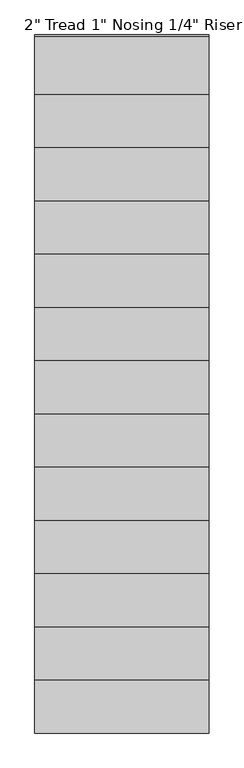
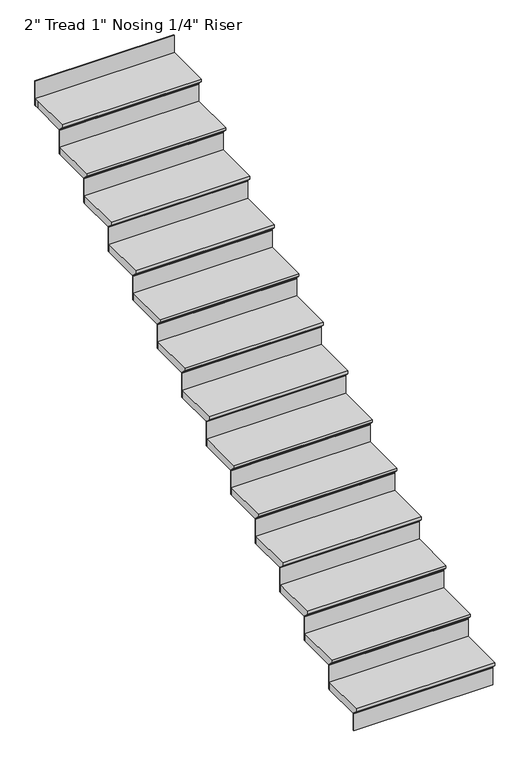
"""IFC4 building model written with IfcOpenShell, lengths in millimetres: stair flight geometry."""

from ifc_helpers import new_model, si_unit, origin, place, context, project, spatial, faceted_brep, source, transform, mapped, element, save


def stair_flight_df872bfd(model_context):
    return source(origin(), model_context, "Body", "Brep", [
        faceted_brep([(-2703.0415084, -23154.3851539, 25384.9005799), (-2703.0415084, -23154.3851539, 25403.9505799), (-3617.4415084, -23154.3851539, 25403.9505799), (-3617.4415084, -23154.3851539, 25384.9005799), (-2703.0415084, -23128.9851539, 25359.5005799), (-3617.4415084, -23128.9851539, 25359.5005799), (-2703.0415084, -22849.5851539, 25403.9505799), (-3617.4415084, -22849.5851539, 25403.9505799), (-3617.4415084, -23128.9851539, 25353.1505799), (-3617.4415084, -22849.5851539, 25353.1505799), (-2703.0415084, -22849.5851539, 25353.1505799), (-2703.0415084, -23128.9851539, 25353.1505799)], [[[0, 1, 2, 3]], [[4, 0, 3, 5]], [[2, 1, 6, 7]], [[8, 9, 10, 11]], [[2, 7, 9, 8, 5, 3]], [[8, 11, 4, 5]], [[6, 1, 0, 4, 11, 10]], [[7, 6, 10, 9]]]),
        faceted_brep([(-2703.0415084, -23128.9851539, 25353.1505799), (-2703.0415084, -23128.9851539, 25234.6172466), (-2703.0415084, -23122.6351539, 25234.6172466), (-2703.0415084, -23122.6351539, 25353.1505799), (-3617.4415084, -23128.9851539, 25353.1505799), (-3617.4415084, -23122.6351539, 25353.1505799), (-3617.4415084, -23122.6351539, 25234.6172466), (-3617.4415084, -23128.9851539, 25234.6172466)], [[[0, 1, 2, 3]], [[4, 5, 6, 7]], [[1, 0, 4, 7]], [[2, 1, 7, 6]], [[3, 2, 6, 5]], [[0, 3, 5, 4]]]),
        faceted_brep([(-2703.0415084, -22849.5851539, 25522.4839133), (-2703.0415084, -22849.5851539, 25353.1505799), (-2703.0415084, -22843.2351539, 25353.1505799), (-2703.0415084, -22843.2351539, 25522.4839133), (-3617.4415084, -22849.5851539, 25522.4839133), (-3617.4415084, -22843.2351539, 25522.4839133), (-3617.4415084, -22843.2351539, 25353.1505799), (-3617.4415084, -22849.5851539, 25353.1505799)], [[[0, 1, 2, 3]], [[4, 5, 6, 7]], [[1, 0, 4, 7]], [[2, 1, 7, 6]], [[3, 2, 6, 5]], [[0, 3, 5, 4]]]),
        faceted_brep([(-3617.4415084, -22874.9851539, 25573.2839133), (-2703.0415084, -22874.9851539, 25573.2839133), (-2703.0415084, -22570.1851539, 25573.2839133), (-3617.4415084, -22570.1851539, 25573.2839133), (-3617.4415084, -22849.5851539, 25522.4839133), (-3617.4415084, -22570.1851539, 25522.4839133), (-2703.0415084, -22570.1851539, 25522.4839133), (-2703.0415084, -22849.5851539, 25522.4839133), (-3617.4415084, -22849.5851539, 25528.8339133), (-3617.4415084, -22874.9851539, 25554.2339133), (-2703.0415084, -22849.5851539, 25528.8339133), (-2703.0415084, -22874.9851539, 25554.2339133)], [[[0, 1, 2, 3]], [[4, 5, 6, 7]], [[0, 3, 5, 4, 8, 9]], [[4, 7, 10, 8]], [[2, 1, 11, 10, 7, 6]], [[3, 2, 6, 5]], [[11, 1, 0, 9]], [[10, 11, 9, 8]]]),
        faceted_brep([(-2703.0415084, -22570.1851539, 25691.8172466), (-2703.0415084, -22570.1851539, 25522.4839133), (-2703.0415084, -22563.8351539, 25522.4839133), (-2703.0415084, -22563.8351539, 25691.8172466), (-3617.4415084, -22570.1851539, 25691.8172466), (-3617.4415084, -22563.8351539, 25691.8172466), (-3617.4415084, -22563.8351539, 25522.4839133), (-3617.4415084, -22570.1851539, 25522.4839133)], [[[0, 1, 2, 3]], [[4, 5, 6, 7]], [[1, 0, 4, 7]], [[2, 1, 7, 6]], [[3, 2, 6, 5]], [[0, 3, 5, 4]]]),
        faceted_brep([(-3617.4415084, -22595.5851539, 25742.6172466), (-2703.0415084, -22595.5851539, 25742.6172466), (-2703.0415084, -22290.7851539, 25742.6172466), (-3617.4415084, -22290.7851539, 25742.6172466), (-3617.4415084, -22570.1851539, 25691.8172466), (-3617.4415084, -22290.7851539, 25691.8172466), (-2703.0415084, -22290.7851539, 25691.8172466), (-2703.0415084, -22570.1851539, 25691.8172466), (-3617.4415084, -22570.1851539, 25698.1672466), (-3617.4415084, -22595.5851539, 25723.5672466), (-2703.0415084, -22570.1851539, 25698.1672466), (-2703.0415084, -22595.5851539, 25723.5672466)], [[[0, 1, 2, 3]], [[4, 5, 6, 7]], [[0, 3, 5, 4, 8, 9]], [[4, 7, 10, 8]], [[2, 1, 11, 10, 7, 6]], [[3, 2, 6, 5]], [[11, 1, 0, 9]], [[10, 11, 9, 8]]]),
        faceted_brep([(-2703.0415084, -22290.7851539, 25861.1505799), (-2703.0415084, -22290.7851539, 25691.8172466), (-2703.0415084, -22284.4351539, 25691.8172466), (-2703.0415084, -22284.4351539, 25861.1505799), (-3617.4415084, -22290.7851539, 25861.1505799), (-3617.4415084, -22284.4351539, 25861.1505799), (-3617.4415084, -22284.4351539, 25691.8172466), (-3617.4415084, -22290.7851539, 25691.8172466)], [[[0, 1, 2, 3]], [[4, 5, 6, 7]], [[1, 0, 4, 7]], [[2, 1, 7, 6]], [[3, 2, 6, 5]], [[0, 3, 5, 4]]]),
        faceted_brep([(-3617.4415084, -22316.1851539, 25911.9505799), (-2703.0415084, -22316.1851539, 25911.9505799), (-2703.0415084, -22011.3851539, 25911.9505799), (-3617.4415084, -22011.3851539, 25911.9505799), (-3617.4415084, -22290.7851539, 25861.1505799), (-3617.4415084, -22011.3851539, 25861.1505799), (-2703.0415084, -22011.3851539, 25861.1505799), (-2703.0415084, -22290.7851539, 25861.1505799), (-3617.4415084, -22290.7851539, 25867.5005799), (-3617.4415084, -22316.1851539, 25892.9005799), (-2703.0415084, -22290.7851539, 25867.5005799), (-2703.0415084, -22316.1851539, 25892.9005799)], [[[0, 1, 2, 3]], [[4, 5, 6, 7]], [[0, 3, 5, 4, 8, 9]], [[4, 7, 10, 8]], [[2, 1, 11, 10, 7, 6]], [[3, 2, 6, 5]], [[11, 1, 0, 9]], [[10, 11, 9, 8]]]),
        faceted_brep([(-2703.0415084, -22011.3851539, 26030.4839133), (-2703.0415084, -22011.3851539, 25861.1505799), (-2703.0415084, -22005.0351539, 25861.1505799), (-2703.0415084, -22005.0351539, 26030.4839133), (-3617.4415084, -22011.3851539, 26030.4839133), (-3617.4415084, -22005.0351539, 26030.4839133), (-3617.4415084, -22005.0351539, 25861.1505799), (-3617.4415084, -22011.3851539, 25861.1505799)], [[[0, 1, 2, 3]], [[4, 5, 6, 7]], [[1, 0, 4, 7]], [[2, 1, 7, 6]], [[3, 2, 6, 5]], [[0, 3, 5, 4]]]),
        faceted_brep([(-3617.4415084, -22036.7851539, 26081.2839133), (-2703.0415084, -22036.7851539, 26081.2839133), (-2703.0415084, -21731.9851539, 26081.2839133), (-3617.4415084, -21731.9851539, 26081.2839133), (-3617.4415084, -22011.3851539, 26030.4839133), (-3617.4415084, -21731.9851539, 26030.4839133), (-2703.0415084, -21731.9851539, 26030.4839133), (-2703.0415084, -22011.3851539, 26030.4839133), (-3617.4415084, -22011.3851539, 26036.8339133), (-3617.4415084, -22036.7851539, 26062.2339133), (-2703.0415084, -22011.3851539, 26036.8339133), (-2703.0415084, -22036.7851539, 26062.2339133)], [[[0, 1, 2, 3]], [[4, 5, 6, 7]], [[0, 3, 5, 4, 8, 9]], [[4, 7, 10, 8]], [[2, 1, 11, 10, 7, 6]], [[3, 2, 6, 5]], [[11, 1, 0, 9]], [[10, 11, 9, 8]]]),
        faceted_brep([(-2703.0415084, -21731.9851539, 26199.8172466), (-2703.0415084, -21731.9851539, 26030.4839133), (-2703.0415084, -21725.6351539, 26030.4839133), (-2703.0415084, -21725.6351539, 26199.8172466), (-3617.4415084, -21731.9851539, 26199.8172466), (-3617.4415084, -21725.6351539, 26199.8172466), (-3617.4415084, -21725.6351539, 26030.4839133), (-3617.4415084, -21731.9851539, 26030.4839133)], [[[0, 1, 2, 3]], [[4, 5, 6, 7]], [[1, 0, 4, 7]], [[2, 1, 7, 6]], [[3, 2, 6, 5]], [[0, 3, 5, 4]]]),
        faceted_brep([(-3617.4415084, -21757.3851539, 26250.6172466), (-2703.0415084, -21757.3851539, 26250.6172466), (-2703.0415084, -21452.5851539, 26250.6172466), (-3617.4415084, -21452.5851539, 26250.6172466), (-3617.4415084, -21731.9851539, 26199.8172466), (-3617.4415084, -21452.5851539, 26199.8172466), (-2703.0415084, -21452.5851539, 26199.8172466), (-2703.0415084, -21731.9851539, 26199.8172466), (-3617.4415084, -21731.9851539, 26206.1672466), (-3617.4415084, -21757.3851539, 26231.5672466), (-2703.0415084, -21731.9851539, 26206.1672466), (-2703.0415084, -21757.3851539, 26231.5672466)], [[[0, 1, 2, 3]], [[4, 5, 6, 7]], [[0, 3, 5, 4, 8, 9]], [[4, 7, 10, 8]], [[2, 1, 11, 10, 7, 6]], [[3, 2, 6, 5]], [[11, 1, 0, 9]], [[10, 11, 9, 8]]]),
        faceted_brep([(-2703.0415084, -21452.5851539, 26369.1505799), (-2703.0415084, -21452.5851539, 26199.8172466), (-2703.0415084, -21446.2351539, 26199.8172466), (-2703.0415084, -21446.2351539, 26369.1505799), (-3617.4415084, -21452.5851539, 26369.1505799), (-3617.4415084, -21446.2351539, 26369.1505799), (-3617.4415084, -21446.2351539, 26199.8172466), (-3617.4415084, -21452.5851539, 26199.8172466)], [[[0, 1, 2, 3]], [[4, 5, 6, 7]], [[1, 0, 4, 7]], [[2, 1, 7, 6]], [[3, 2, 6, 5]], [[0, 3, 5, 4]]]),
        faceted_brep([(-3617.4415084, -21477.9851539, 26419.9505799), (-2703.0415084, -21477.9851539, 26419.9505799), (-2703.0415084, -21173.1851539, 26419.9505799), (-3617.4415084, -21173.1851539, 26419.9505799), (-3617.4415084, -21452.5851539, 26369.1505799), (-3617.4415084, -21173.1851539, 26369.1505799), (-2703.0415084, -21173.1851539, 26369.1505799), (-2703.0415084, -21452.5851539, 26369.1505799), (-3617.4415084, -21452.5851539, 26375.5005799), (-3617.4415084, -21477.9851539, 26400.9005799), (-2703.0415084, -21452.5851539, 26375.5005799), (-2703.0415084, -21477.9851539, 26400.9005799)], [[[0, 1, 2, 3]], [[4, 5, 6, 7]], [[0, 3, 5, 4, 8, 9]], [[4, 7, 10, 8]], [[2, 1, 11, 10, 7, 6]], [[3, 2, 6, 5]], [[11, 1, 0, 9]], [[10, 11, 9, 8]]]),
        faceted_brep([(-2703.0415084, -21173.1851539, 26538.4839133), (-2703.0415084, -21173.1851539, 26369.1505799), (-2703.0415084, -21166.8351539, 26369.1505799), (-2703.0415084, -21166.8351539, 26538.4839133), (-3617.4415084, -21173.1851539, 26538.4839133), (-3617.4415084, -21166.8351539, 26538.4839133), (-3617.4415084, -21166.8351539, 26369.1505799), (-3617.4415084, -21173.1851539, 26369.1505799)], [[[0, 1, 2, 3]], [[4, 5, 6, 7]], [[1, 0, 4, 7]], [[2, 1, 7, 6]], [[3, 2, 6, 5]], [[0, 3, 5, 4]]]),
        faceted_brep([(-3617.4415084, -21198.5851539, 26589.2839133), (-2703.0415084, -21198.5851539, 26589.2839133), (-2703.0415084, -20893.7851539, 26589.2839133), (-3617.4415084, -20893.7851539, 26589.2839133), (-3617.4415084, -21173.1851539, 26538.4839133), (-3617.4415084, -20893.7851539, 26538.4839133), (-2703.0415084, -20893.7851539, 26538.4839133), (-2703.0415084, -21173.1851539, 26538.4839133), (-3617.4415084, -21173.1851539, 26544.8339133), (-3617.4415084, -21198.5851539, 26570.2339133), (-2703.0415084, -21173.1851539, 26544.8339133), (-2703.0415084, -21198.5851539, 26570.2339133)], [[[0, 1, 2, 3]], [[4, 5, 6, 7]], [[0, 3, 5, 4, 8, 9]], [[4, 7, 10, 8]], [[2, 1, 11, 10, 7, 6]], [[3, 2, 6, 5]], [[11, 1, 0, 9]], [[10, 11, 9, 8]]]),
        faceted_brep([(-2703.0415084, -20893.7851539, 26707.8172466), (-2703.0415084, -20893.7851539, 26538.4839133), (-2703.0415084, -20887.4351539, 26538.4839133), (-2703.0415084, -20887.4351539, 26707.8172466), (-3617.4415084, -20893.7851539, 26707.8172466), (-3617.4415084, -20887.4351539, 26707.8172466), (-3617.4415084, -20887.4351539, 26538.4839133), (-3617.4415084, -20893.7851539, 26538.4839133)], [[[0, 1, 2, 3]], [[4, 5, 6, 7]], [[1, 0, 4, 7]], [[2, 1, 7, 6]], [[3, 2, 6, 5]], [[0, 3, 5, 4]]]),
        faceted_brep([(-3617.4415084, -20919.1851539, 26758.6172466), (-2703.0415084, -20919.1851539, 26758.6172466), (-2703.0415084, -20614.3851539, 26758.6172466), (-3617.4415084, -20614.3851539, 26758.6172466), (-3617.4415084, -20893.7851539, 26707.8172466), (-3617.4415084, -20614.3851539, 26707.8172466), (-2703.0415084, -20614.3851539, 26707.8172466), (-2703.0415084, -20893.7851539, 26707.8172466), (-3617.4415084, -20893.7851539, 26714.1672466), (-3617.4415084, -20919.1851539, 26739.5672466), (-2703.0415084, -20893.7851539, 26714.1672466), (-2703.0415084, -20919.1851539, 26739.5672466)], [[[0, 1, 2, 3]], [[4, 5, 6, 7]], [[0, 3, 5, 4, 8, 9]], [[4, 7, 10, 8]], [[2, 1, 11, 10, 7, 6]], [[3, 2, 6, 5]], [[11, 1, 0, 9]], [[10, 11, 9, 8]]]),
        faceted_brep([(-2703.0415084, -20614.3851539, 26877.1505799), (-2703.0415084, -20614.3851539, 26707.8172466), (-2703.0415084, -20608.0351539, 26707.8172466), (-2703.0415084, -20608.0351539, 26877.1505799), (-3617.4415084, -20614.3851539, 26877.1505799), (-3617.4415084, -20608.0351539, 26877.1505799), (-3617.4415084, -20608.0351539, 26707.8172466), (-3617.4415084, -20614.3851539, 26707.8172466)], [[[0, 1, 2, 3]], [[4, 5, 6, 7]], [[1, 0, 4, 7]], [[2, 1, 7, 6]], [[3, 2, 6, 5]], [[0, 3, 5, 4]]]),
        faceted_brep([(-3617.4415084, -20639.7851539, 26927.9505799), (-2703.0415084, -20639.7851539, 26927.9505799), (-2703.0415084, -20334.9851539, 26927.9505799), (-3617.4415084, -20334.9851539, 26927.9505799), (-3617.4415084, -20614.3851539, 26877.1505799), (-3617.4415084, -20334.9851539, 26877.1505799), (-2703.0415084, -20334.9851539, 26877.1505799), (-2703.0415084, -20614.3851539, 26877.1505799), (-3617.4415084, -20614.3851539, 26883.5005799), (-3617.4415084, -20639.7851539, 26908.9005799), (-2703.0415084, -20614.3851539, 26883.5005799), (-2703.0415084, -20639.7851539, 26908.9005799)], [[[0, 1, 2, 3]], [[4, 5, 6, 7]], [[0, 3, 5, 4, 8, 9]], [[4, 7, 10, 8]], [[2, 1, 11, 10, 7, 6]], [[3, 2, 6, 5]], [[11, 1, 0, 9]], [[10, 11, 9, 8]]]),
        faceted_brep([(-2703.0415084, -20334.9851539, 27046.4839133), (-2703.0415084, -20334.9851539, 26877.1505799), (-2703.0415084, -20328.6351539, 26877.1505799), (-2703.0415084, -20328.6351539, 27046.4839133), (-3617.4415084, -20334.9851539, 27046.4839133), (-3617.4415084, -20328.6351539, 27046.4839133), (-3617.4415084, -20328.6351539, 26877.1505799), (-3617.4415084, -20334.9851539, 26877.1505799)], [[[0, 1, 2, 3]], [[4, 5, 6, 7]], [[1, 0, 4, 7]], [[2, 1, 7, 6]], [[3, 2, 6, 5]], [[0, 3, 5, 4]]]),
        faceted_brep([(-3617.4415084, -20360.3851539, 27097.2839133), (-2703.0415084, -20360.3851539, 27097.2839133), (-2703.0415084, -20055.5851539, 27097.2839133), (-3617.4415084, -20055.5851539, 27097.2839133), (-3617.4415084, -20334.9851539, 27046.4839133), (-3617.4415084, -20055.5851539, 27046.4839133), (-2703.0415084, -20055.5851539, 27046.4839133), (-2703.0415084, -20334.9851539, 27046.4839133), (-3617.4415084, -20334.9851539, 27052.8339133), (-3617.4415084, -20360.3851539, 27078.2339133), (-2703.0415084, -20334.9851539, 27052.8339133), (-2703.0415084, -20360.3851539, 27078.2339133)], [[[0, 1, 2, 3]], [[4, 5, 6, 7]], [[0, 3, 5, 4, 8, 9]], [[4, 7, 10, 8]], [[2, 1, 11, 10, 7, 6]], [[3, 2, 6, 5]], [[11, 1, 0, 9]], [[10, 11, 9, 8]]]),
        faceted_brep([(-2703.0415084, -20055.5851539, 27215.8172466), (-2703.0415084, -20055.5851539, 27046.4839133), (-2703.0415084, -20049.2351539, 27046.4839133), (-2703.0415084, -20049.2351539, 27215.8172466), (-3617.4415084, -20055.5851539, 27215.8172466), (-3617.4415084, -20049.2351539, 27215.8172466), (-3617.4415084, -20049.2351539, 27046.4839133), (-3617.4415084, -20055.5851539, 27046.4839133)], [[[0, 1, 2, 3]], [[4, 5, 6, 7]], [[1, 0, 4, 7]], [[2, 1, 7, 6]], [[3, 2, 6, 5]], [[0, 3, 5, 4]]]),
        faceted_brep([(-3617.4415084, -20080.9851539, 27266.6172466), (-2703.0415084, -20080.9851539, 27266.6172466), (-2703.0415084, -19776.1851539, 27266.6172466), (-3617.4415084, -19776.1851539, 27266.6172466), (-3617.4415084, -20055.5851539, 27215.8172466), (-3617.4415084, -19776.1851539, 27215.8172466), (-2703.0415084, -19776.1851539, 27215.8172466), (-2703.0415084, -20055.5851539, 27215.8172466), (-3617.4415084, -20055.5851539, 27222.1672466), (-3617.4415084, -20080.9851539, 27247.5672466), (-2703.0415084, -20055.5851539, 27222.1672466), (-2703.0415084, -20080.9851539, 27247.5672466)], [[[0, 1, 2, 3]], [[4, 5, 6, 7]], [[0, 3, 5, 4, 8, 9]], [[4, 7, 10, 8]], [[2, 1, 11, 10, 7, 6]], [[3, 2, 6, 5]], [[11, 1, 0, 9]], [[10, 11, 9, 8]]]),
        faceted_brep([(-2703.0415084, -19496.7851539, 27554.4839133), (-2703.0415084, -19496.7851539, 27385.1505799), (-2703.0415084, -19490.4351539, 27385.1505799), (-2703.0415084, -19490.4351539, 27554.4839133), (-3617.4415084, -19496.7851539, 27554.4839133), (-3617.4415084, -19490.4351539, 27554.4839133), (-3617.4415084, -19490.4351539, 27385.1505799), (-3617.4415084, -19496.7851539, 27385.1505799)], [[[0, 1, 2, 3]], [[4, 5, 6, 7]], [[1, 0, 4, 7]], [[2, 1, 7, 6]], [[3, 2, 6, 5]], [[0, 3, 5, 4]]]),
        faceted_brep([(-2703.0415084, -19776.1851539, 27385.1505799), (-2703.0415084, -19776.1851539, 27215.8172466), (-2703.0415084, -19769.8351539, 27215.8172466), (-2703.0415084, -19769.8351539, 27385.1505799), (-3617.4415084, -19776.1851539, 27385.1505799), (-3617.4415084, -19769.8351539, 27385.1505799), (-3617.4415084, -19769.8351539, 27215.8172466), (-3617.4415084, -19776.1851539, 27215.8172466)], [[[0, 1, 2, 3]], [[4, 5, 6, 7]], [[1, 0, 4, 7]], [[2, 1, 7, 6]], [[3, 2, 6, 5]], [[0, 3, 5, 4]]]),
        faceted_brep([(-3617.4415084, -19496.7851539, 27435.9505799), (-3617.4415084, -19522.1851539, 27435.9505799), (-3617.4415084, -19801.5851539, 27435.9505799), (-2703.0415084, -19801.5851539, 27435.9505799), (-2703.0415084, -19496.7851539, 27435.9505799), (-3617.4415084, -19522.1851539, 27385.1505799), (-3617.4415084, -19496.7851539, 27385.1505799), (-2703.0415084, -19496.7851539, 27385.1505799), (-2703.0415084, -19776.1851539, 27385.1505799), (-3617.4415084, -19776.1851539, 27385.1505799), (-3617.4415084, -19776.1851539, 27391.5005799), (-3617.4415084, -19801.5851539, 27416.9005799), (-2703.0415084, -19776.1851539, 27391.5005799), (-2703.0415084, -19801.5851539, 27416.9005799)], [[[0, 1, 2, 3, 4]], [[5, 6, 7, 8, 9]], [[1, 0, 6, 5]], [[2, 1, 5, 9, 10, 11]], [[9, 8, 12, 10]], [[4, 3, 13, 12, 8, 7]], [[0, 4, 7, 6]], [[13, 3, 2, 11]], [[12, 13, 11, 10]]]),
    ])


if __name__ == "__main__":
    model = new_model("IFC4")
    model_context = context("Model", 3, world=origin())
    ifc_project = project(units=[si_unit("LENGTHUNIT", "METRE", prefix="MILLI")], contexts=[model_context])
    site = spatial("IfcSite", under=ifc_project)
    building = spatial("IfcBuilding", under=site)
    placement = place(None, origin())
    stair_flight_shape = stair_flight_df872bfd(model_context)
    element("IfcStairFlight", 1, ObjectType="2\" Tread 1\" Nosing 1/4\" Riser", at=placement, inside=building, context=model_context, shape_type="MappedRepresentation", body=[
        mapped(stair_flight_shape, transform((0.0, 0.0, 0.0), x_axis=(1.0, 0.0, 0.0), y_axis=(0.0, 1.0, 0.0), z_axis=(0.0, 0.0, 1.0))),
    ])
    save(model, "model.ifc")
